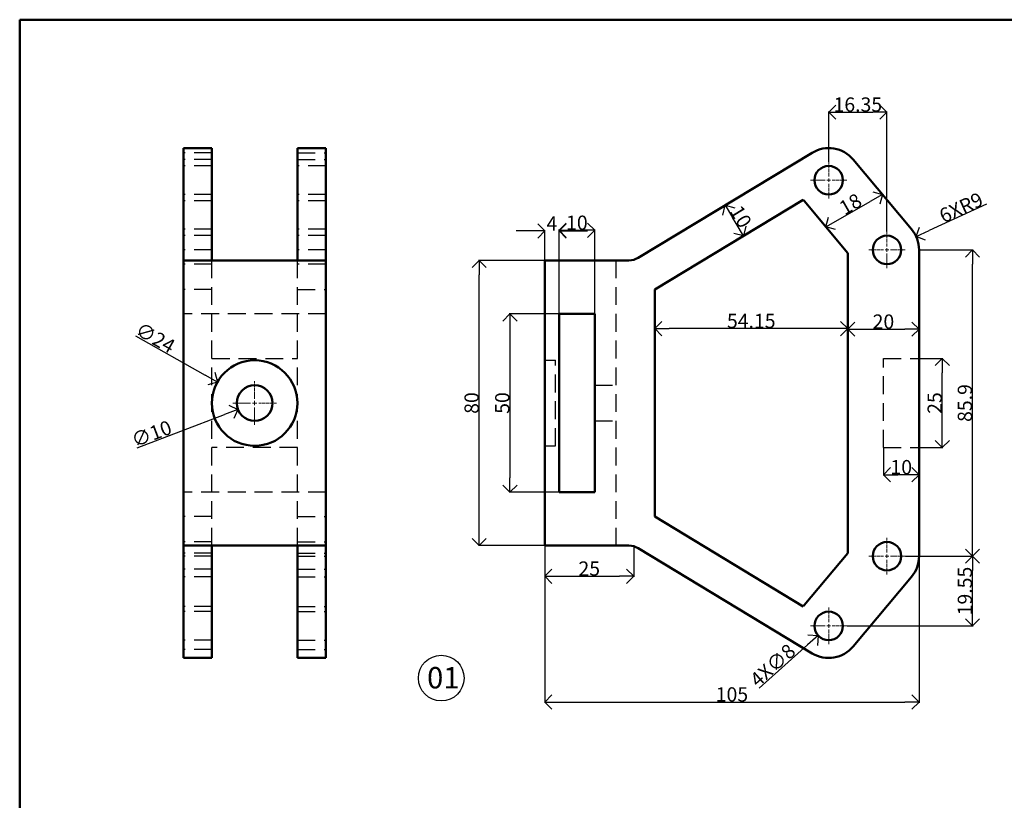
# Model space of a CAD drawing. Units: millimetres. Extents: x 45 to 546, y 51 to 638.
# Tile 3 of 4: x 45 to 322, y 419 to 638. Entities that reach past the tile are written whole.
import ezdxf

# ---------------------------------------------------------------- set-up
doc = ezdxf.new("R2010")
doc.units = ezdxf.units.MM
doc.header["$MEASUREMENT"] = 0
doc.linetypes.add('CENTER2', pattern=[1.125, 0.75, -0.125, 0.125, -0.125])
doc.linetypes.add('HIDDEN', pattern=[0.375, 0.25, -0.125])
for name, color, linetype, lineweight in [('M-CNTR', 1, 'CENTER2', 18), ('M-DIMS', 2, 'Continuous', 25), ('M-HIDN', 8, 'HIDDEN', 25), ('M-OUTL', 7, 'Continuous', 50), ('M-TEXT', 7, 'Continuous', 25), ('M-TTLB', 7, 'Continuous', 50)]:
    doc.layers.add(name, color=color, linetype=linetype, lineweight=lineweight)
doc.styles.get("Standard").update_dxf_attribs({"font": 'arial.ttf'})
doc.dimstyles.get("Standard").update_dxf_attribs({"dimtxt": 4, "dimasz": 4, "dimexe": 0.18, "dimexo": 0.0625, "dimgap": 0.09, "dimtad": 1, "dimdec": 0, "dimzin": 0, "dimdsep": 46, "dimtxsty": 'Standard', "dimblk": 'OPEN90', "dimcen": 0.09, "dimclre": 251, "dimadec": 0, "dimazin": 0, "dimtfac": 1, "dimtdec": 0, "dimtofl": 0, "dimtmove": 0, "dimatfit": 3, "dimfxl": 1, "dimtolj": 1, "dimtzin": 0, "dimarcsym": 0})

# ---------------------------------------------------------------- blocks, each defined once
blk = doc.blocks.new('*U4')
at = {"layer": 'M-CNTR', "color": 0, "transparency": 16777216}
for p, q in [((0, 1.2), (0, 6.12)), ((-6.12, 0), (-1.2, 0)), ((1.2, 0), (6.12, 0)), ((0, -6.12), (0, -1.2))]:
    blk.add_line(p, q, dxfattribs=at)
at = {"layer": 'M-CNTR', "color": 0, "linetype": 'Continuous', "transparency": 16777216}
for p, q in [((-0.6, 0), (0.6, 0)), ((0, -0.6), (0, 0.6))]:
    blk.add_line(p, q, dxfattribs=at)
blk = doc.blocks.new('*U5')
at = {"layer": 'M-CNTR', "color": 0, "transparency": 16777216}
for p, q in [((0, 1), (0, 5.12)), ((-5.12, 0), (-1, 0)), ((1, 0), (5.12, 0)), ((0, -5.12), (0, -1))]:
    blk.add_line(p, q, dxfattribs=at)
at = {"layer": 'M-CNTR', "color": 0, "linetype": 'Continuous', "transparency": 16777216}
for p, q in [((-0.5, 0), (0.5, 0)), ((0, -0.5), (0, 0.5))]:
    blk.add_line(p, q, dxfattribs=at)
blk = doc.blocks.new('*U6')
at = {"layer": 'M-CNTR', "color": 0, "transparency": 16777216}
for p, q in [((0, 1), (0, 5.12)), ((-5.12, 0), (-1, 0)), ((1, 0), (5.12, 0)), ((0, -5.12), (0, -1))]:
    blk.add_line(p, q, dxfattribs=at)
at = {"layer": 'M-CNTR', "color": 0, "linetype": 'Continuous', "transparency": 16777216}
for p, q in [((-0.5, 0), (0.5, 0)), ((0, -0.5), (0, 0.5))]:
    blk.add_line(p, q, dxfattribs=at)
blk = doc.blocks.new('*U7')
at = {"layer": 'M-CNTR', "color": 0, "transparency": 16777216}
for p, q in [((0, 1), (0, 5.12)), ((-5.12, 0), (-1, 0)), ((1, 0), (5.12, 0)), ((0, -5.12), (0, -1))]:
    blk.add_line(p, q, dxfattribs=at)
at = {"layer": 'M-CNTR', "color": 0, "linetype": 'Continuous', "transparency": 16777216}
for p, q in [((-0.5, 0), (0.5, 0)), ((0, -0.5), (0, 0.5))]:
    blk.add_line(p, q, dxfattribs=at)
blk = doc.blocks.new('*U8')
at = {"layer": 'M-CNTR', "color": 0, "transparency": 16777216}
for p, q in [((0, 1), (0, 5.12)), ((-5.12, 0), (-1, 0)), ((1, 0), (5.12, 0)), ((0, -5.12), (0, -1))]:
    blk.add_line(p, q, dxfattribs=at)
at = {"layer": 'M-CNTR', "color": 0, "linetype": 'Continuous', "transparency": 16777216}
for p, q in [((-0.5, 0), (0.5, 0)), ((0, -0.5), (0, 0.5))]:
    blk.add_line(p, q, dxfattribs=at)
blk = doc.blocks.new('_Open90')
at = {"color": 0, "linetype": 'ByBlock', "lineweight": -2}
for p, q in [((0, 0), (-1, 0)), ((-0.5, 0.5), (0, 0)), ((0, 0), (-0.5, -0.5))]:
    blk.add_line(p, q, dxfattribs=at)
blk = doc.blocks.new('*D9')
at = {"layer": 'Defpoints', "color": 0, "transparency": 16777216}
for p in [(100.83, 536.27), (121.73, 524.47)]:
    blk.add_point(p, dxfattribs=at)
at = {"layer": 'M-DIMS', "color": 0, "lineweight": -2, "transparency": 16777216}
for p, q in [((77.85, 549.25), (97.35, 538.24)), ((111.28, 530.28), (111.28, 530.46)), ((111.19, 530.37), (111.37, 530.37))]:
    blk.add_line(p, q, dxfattribs=at)
at = {"layer": 'M-DIMS', "color": 0, "lineweight": -2, "transparency": 16777216, "xscale": 4, "yscale": 4, "zscale": 4, "rotation": 330.5336294164444}
blk.add_blockref('_Open90', (100.83, 536.27), dxfattribs=at)
at = {"layer": 'M-DIMS', "color": 0, "transparency": 16777216, "insert": (83.42, 548.69), "char_height": 4, "attachment_point": 5, "rotation": 330.5336}
blk.add_mtext('\\A1;∅24', dxfattribs=at)
blk = doc.blocks.new('*D10')
at = {"layer": 'Defpoints', "color": 0, "transparency": 16777216}
for p in [(115.95, 532.14), (106.6, 528.59)]:
    blk.add_point(p, dxfattribs=at)
at = {"layer": 'M-DIMS', "color": 0, "lineweight": -2, "transparency": 16777216}
for p, q in [((111.28, 530.28), (111.28, 530.46)), ((111.19, 530.37), (111.37, 530.37)), ((78.35, 517.86), (102.86, 527.17))]:
    blk.add_line(p, q, dxfattribs=at)
at = {"layer": 'M-DIMS', "color": 0, "lineweight": -2, "transparency": 16777216, "xscale": 4, "yscale": 4, "zscale": 4, "rotation": 20.80031859419077}
blk.add_blockref('_Open90', (106.6, 528.59), dxfattribs=at)
at = {"layer": 'M-DIMS', "color": 0, "transparency": 16777216, "insert": (82.34, 521.78), "char_height": 4, "attachment_point": 5, "rotation": 20.8003}
blk.add_mtext('\\A1;∅10', dxfattribs=at)
blk = doc.blocks.new('*D11')
at = {"layer": 'Defpoints', "color": 0, "transparency": 16777216}
for p in [(174.27, 570.38), (192.68, 570.38), (192.68, 490.38)]:
    blk.add_point(p, dxfattribs=at)
at = {"layer": 'M-DIMS', "color": 0, "lineweight": -2, "transparency": 16777216}
for p, q in [((192.61, 570.38), (174.09, 570.38)), ((174.27, 494.38), (174.27, 566.38)), ((192.61, 490.38), (174.09, 490.38))]:
    blk.add_line(p, q, dxfattribs=at)
at = {"layer": 'M-DIMS', "color": 0, "lineweight": -2, "transparency": 16777216, "xscale": 4, "yscale": 4, "zscale": 4}
for p, rotation in [((174.27, 570.38), 90), ((174.27, 490.38), 270)]:
    blk.add_blockref('_Open90', p, dxfattribs=dict(at, rotation=rotation))
at = {"layer": 'M-DIMS', "color": 0, "transparency": 16777216, "insert": (172.14, 530.38), "char_height": 4, "attachment_point": 5, "rotation": 90}
blk.add_mtext('\\A1;80', dxfattribs=at)
blk = doc.blocks.new('*D12')
at = {"layer": 'Defpoints', "color": 0, "transparency": 16777216}
for p in [(196.68, 555.38), (182.88, 505.38), (196.68, 505.38)]:
    blk.add_point(p, dxfattribs=at)
at = {"layer": 'M-DIMS', "color": 0, "lineweight": -2, "transparency": 16777216}
for p, q in [((196.61, 555.38), (182.7, 555.38)), ((182.88, 551.38), (182.88, 509.38)), ((196.61, 505.38), (182.7, 505.38))]:
    blk.add_line(p, q, dxfattribs=at)
at = {"layer": 'M-DIMS', "color": 0, "lineweight": -2, "transparency": 16777216, "xscale": 4, "yscale": 4, "zscale": 4}
for p, rotation in [((182.88, 555.38), 90), ((182.88, 505.38), 270)]:
    blk.add_blockref('_Open90', p, dxfattribs=dict(at, rotation=rotation))
at = {"layer": 'M-DIMS', "color": 0, "transparency": 16777216, "insert": (180.75, 530.38), "char_height": 4, "attachment_point": 5, "rotation": 90}
blk.add_mtext('\\A1;50', dxfattribs=at)
blk = doc.blocks.new('*D13')
at = {"layer": 'Defpoints', "color": 0, "transparency": 16777216}
for p in [(192.68, 578.65), (192.68, 570.38), (196.68, 555.38)]:
    blk.add_point(p, dxfattribs=at)
at = {"layer": 'M-DIMS', "color": 0, "lineweight": -2, "transparency": 16777216}
for p, q in [((188.68, 578.65), (184.68, 578.65)), ((192.68, 570.44), (192.68, 578.83)), ((196.68, 555.44), (196.68, 578.83)), ((200.68, 578.65), (204.68, 578.65))]:
    blk.add_line(p, q, dxfattribs=at)
at = {"layer": 'M-DIMS', "color": 0, "lineweight": -2, "transparency": 16777216, "xscale": 4, "yscale": 4, "zscale": 4}
blk.add_blockref('_Open90', (192.68, 578.65), dxfattribs=at)
at = {"layer": 'M-DIMS', "color": 0, "lineweight": -2, "transparency": 16777216, "xscale": 4, "yscale": 4, "zscale": 4, "rotation": 180}
blk.add_blockref('_Open90', (196.68, 578.65), dxfattribs=at)
at = {"layer": 'M-DIMS', "color": 0, "transparency": 16777216, "insert": (194.68, 580.74), "char_height": 4, "attachment_point": 5}
blk.add_mtext('\\A1;4', dxfattribs=at)
blk = doc.blocks.new('*D14')
at = {"layer": 'Defpoints', "color": 0, "transparency": 16777216}
for p in [(206.68, 578.83), (196.68, 555.38), (206.68, 555.38)]:
    blk.add_point(p, dxfattribs=at)
at = {"layer": 'M-DIMS', "color": 0, "lineweight": -2, "transparency": 16777216}
for p, q in [((196.68, 555.44), (196.68, 579.01)), ((200.68, 578.83), (202.68, 578.83)), ((206.68, 555.44), (206.68, 579.01))]:
    blk.add_line(p, q, dxfattribs=at)
at = {"layer": 'M-DIMS', "color": 0, "lineweight": -2, "transparency": 16777216, "xscale": 4, "yscale": 4, "zscale": 4, "rotation": 180}
blk.add_blockref('_Open90', (196.68, 578.83), dxfattribs=at)
at = {"layer": 'M-DIMS', "color": 0, "lineweight": -2, "transparency": 16777216, "xscale": 4, "yscale": 4, "zscale": 4}
blk.add_blockref('_Open90', (206.68, 578.83), dxfattribs=at)
at = {"layer": 'M-DIMS', "color": 0, "transparency": 16777216, "insert": (201.68, 580.96), "char_height": 4, "attachment_point": 5}
blk.add_mtext('\\A1;10', dxfattribs=at)
blk = doc.blocks.new('*D15')
at = {"layer": 'Defpoints', "color": 0, "transparency": 16777216}
for p in [(288.68, 611.96), (272.33, 598), (288.68, 578.45)]:
    blk.add_point(p, dxfattribs=at)
at = {"layer": 'M-DIMS', "color": 0, "lineweight": -2, "transparency": 16777216}
for p, q in [((272.33, 598.06), (272.33, 612.14)), ((276.33, 611.96), (284.68, 611.96)), ((288.68, 578.51), (288.68, 612.14))]:
    blk.add_line(p, q, dxfattribs=at)
at = {"layer": 'M-DIMS', "color": 0, "lineweight": -2, "transparency": 16777216, "xscale": 4, "yscale": 4, "zscale": 4, "rotation": 180}
blk.add_blockref('_Open90', (272.33, 611.96), dxfattribs=at)
at = {"layer": 'M-DIMS', "color": 0, "lineweight": -2, "transparency": 16777216, "xscale": 4, "yscale": 4, "zscale": 4}
blk.add_blockref('_Open90', (288.68, 611.96), dxfattribs=at)
at = {"layer": 'M-DIMS', "color": 0, "transparency": 16777216, "insert": (280.5, 614.1), "char_height": 4, "attachment_point": 5}
blk.add_mtext('\\A1;16.35', dxfattribs=at)
blk = doc.blocks.new('*D16')
at = {"layer": 'Defpoints', "color": 0, "transparency": 16777216}
for p in [(243.27, 585.84), (241.76, 584.92), (246.93, 576.36)]:
    blk.add_point(p, dxfattribs=at)
at = {"layer": 'M-DIMS', "color": 0, "lineweight": -2, "transparency": 16777216}
for p, q in [((241.81, 584.96), (243.42, 585.93)), ((246.37, 580.7), (245.34, 582.41)), ((246.98, 576.4), (248.6, 577.37))]:
    blk.add_line(p, q, dxfattribs=at)
at = {"layer": 'M-DIMS', "color": 0, "lineweight": -2, "transparency": 16777216, "xscale": 4, "yscale": 4, "zscale": 4}
for p, rotation in [((243.27, 585.84), 121.1367457519999), ((248.44, 577.28), 301.136745752)]:
    blk.add_blockref('_Open90', p, dxfattribs=dict(at, rotation=rotation))
at = {"layer": 'M-DIMS', "color": 0, "transparency": 16777216, "insert": (247.68, 582.66), "char_height": 4, "attachment_point": 5, "rotation": 301.1367}
blk.add_mtext('\\A1;10', dxfattribs=at)
blk = doc.blocks.new('*D17')
at = {"layer": 'Defpoints', "color": 0, "transparency": 16777216}
for p in [(287.4, 588.88), (287.4, 588.88), (271.55, 579.78)]:
    blk.add_point(p, dxfattribs=at)
at = {"layer": 'M-DIMS', "color": 0, "lineweight": -2, "transparency": 16777216}
for p, q in [((287.44, 588.82), (287.49, 588.72)), ((275.02, 581.77), (283.94, 586.88)), ((271.58, 579.72), (271.64, 579.62))]:
    blk.add_line(p, q, dxfattribs=at)
at = {"layer": 'M-DIMS', "color": 0, "lineweight": -2, "transparency": 16777216, "xscale": 4, "yscale": 4, "zscale": 4}
for p, rotation in [((287.4, 588.88), 29.84897271971798), ((271.55, 579.78), 209.848972719718)]:
    blk.add_blockref('_Open90', p, dxfattribs=dict(at, rotation=rotation))
at = {"layer": 'M-DIMS', "color": 0, "transparency": 16777216, "insert": (278.42, 586.18), "char_height": 4, "attachment_point": 5, "rotation": 29.849}
blk.add_mtext('\\A1;18', dxfattribs=at)
blk = doc.blocks.new('*D18')
at = {"layer": 'Defpoints', "color": 0, "transparency": 16777216}
for p in [(192.68, 490.38), (217.62, 490.19), (217.62, 481.81)]:
    blk.add_point(p, dxfattribs=at)
at = {"layer": 'M-DIMS', "color": 0, "lineweight": -2, "transparency": 16777216}
for p, q in [((192.68, 490.31), (192.68, 481.63)), ((217.62, 490.13), (217.62, 481.63)), ((196.68, 481.81), (213.62, 481.81))]:
    blk.add_line(p, q, dxfattribs=at)
at = {"layer": 'M-DIMS', "color": 0, "lineweight": -2, "transparency": 16777216, "xscale": 4, "yscale": 4, "zscale": 4, "rotation": 180}
blk.add_blockref('_Open90', (192.68, 481.81), dxfattribs=at)
at = {"layer": 'M-DIMS', "color": 0, "lineweight": -2, "transparency": 16777216, "xscale": 4, "yscale": 4, "zscale": 4}
blk.add_blockref('_Open90', (217.62, 481.81), dxfattribs=at)
at = {"layer": 'M-DIMS', "color": 0, "transparency": 16777216, "insert": (205.15, 483.95), "char_height": 4, "attachment_point": 5}
blk.add_mtext('\\A1;25', dxfattribs=at)
blk = doc.blocks.new('*D19')
at = {"layer": 'Defpoints', "color": 0, "transparency": 16777216}
for p in [(192.68, 490.38), (297.68, 487.43), (297.68, 446.52)]:
    blk.add_point(p, dxfattribs=at)
at = {"layer": 'M-DIMS', "color": 0, "lineweight": -2, "transparency": 16777216}
for p, q in [((192.68, 490.31), (192.68, 446.34)), ((297.68, 487.36), (297.68, 446.34)), ((196.68, 446.52), (293.68, 446.52))]:
    blk.add_line(p, q, dxfattribs=at)
at = {"layer": 'M-DIMS', "color": 0, "lineweight": -2, "transparency": 16777216, "xscale": 4, "yscale": 4, "zscale": 4, "rotation": 180}
blk.add_blockref('_Open90', (192.68, 446.52), dxfattribs=at)
at = {"layer": 'M-DIMS', "color": 0, "lineweight": -2, "transparency": 16777216, "xscale": 4, "yscale": 4, "zscale": 4}
blk.add_blockref('_Open90', (297.68, 446.52), dxfattribs=at)
at = {"layer": 'M-DIMS', "color": 0, "transparency": 16777216, "insert": (245.18, 448.65), "char_height": 4, "attachment_point": 5}
blk.add_mtext('\\A1;105', dxfattribs=at)
blk = doc.blocks.new('*D20')
at = {"layer": 'Defpoints', "color": 0, "transparency": 16777216}
for p in [(293.8, 487.43), (312.66, 487.43), (277.45, 467.88)]:
    blk.add_point(p, dxfattribs=at)
at = {"layer": 'M-DIMS', "color": 0, "lineweight": -2, "transparency": 16777216}
for p, q in [((293.86, 487.43), (312.84, 487.43)), ((312.66, 471.88), (312.66, 483.43)), ((277.51, 467.88), (312.84, 467.88))]:
    blk.add_line(p, q, dxfattribs=at)
at = {"layer": 'M-DIMS', "color": 0, "lineweight": -2, "transparency": 16777216, "xscale": 4, "yscale": 4, "zscale": 4}
for p, rotation in [((312.66, 487.43), 90), ((312.66, 467.88), 270)]:
    blk.add_blockref('_Open90', p, dxfattribs=dict(at, rotation=rotation))
at = {"layer": 'M-DIMS', "color": 0, "transparency": 16777216, "insert": (310.53, 477.65), "char_height": 4, "attachment_point": 5, "rotation": 90}
blk.add_mtext('\\A1;19.55', dxfattribs=at)
blk = doc.blocks.new('*D21')
at = {"layer": 'Defpoints', "color": 0, "transparency": 16777216}
for p in [(297.68, 573.33), (312.66, 573.33), (297.68, 487.43)]:
    blk.add_point(p, dxfattribs=at)
at = {"layer": 'M-DIMS', "color": 0, "lineweight": -2, "transparency": 16777216}
for p, q in [((297.74, 573.33), (312.84, 573.33)), ((312.66, 491.43), (312.66, 569.33)), ((297.74, 487.43), (312.84, 487.43))]:
    blk.add_line(p, q, dxfattribs=at)
at = {"layer": 'M-DIMS', "color": 0, "lineweight": -2, "transparency": 16777216, "xscale": 4, "yscale": 4, "zscale": 4}
for p, rotation in [((312.66, 573.33), 90), ((312.66, 487.43), 270)]:
    blk.add_blockref('_Open90', p, dxfattribs=dict(at, rotation=rotation))
at = {"layer": 'M-DIMS', "color": 0, "transparency": 16777216, "insert": (310.53, 530.38), "char_height": 4, "attachment_point": 5, "rotation": 90}
blk.add_mtext('\\A1;85.9', dxfattribs=at)
blk = doc.blocks.new('*D22')
at = {"layer": 'Defpoints', "color": 0, "transparency": 16777216}
for p in [(297.68, 542.88), (304.19, 542.88), (297.68, 517.88)]:
    blk.add_point(p, dxfattribs=at)
at = {"layer": 'M-DIMS', "color": 0, "lineweight": -2, "transparency": 16777216}
for p, q in [((297.74, 542.88), (304.37, 542.88)), ((304.19, 521.88), (304.19, 538.88)), ((297.74, 517.88), (304.37, 517.88))]:
    blk.add_line(p, q, dxfattribs=at)
at = {"layer": 'M-DIMS', "color": 0, "lineweight": -2, "transparency": 16777216, "xscale": 4, "yscale": 4, "zscale": 4}
for p, rotation in [((304.19, 542.88), 90), ((304.19, 517.88), 270)]:
    blk.add_blockref('_Open90', p, dxfattribs=dict(at, rotation=rotation))
at = {"layer": 'M-DIMS', "color": 0, "transparency": 16777216, "insert": (302.06, 530.38), "char_height": 4, "attachment_point": 5, "rotation": 90}
blk.add_mtext('\\A1;25', dxfattribs=at)
blk = doc.blocks.new('*D23')
at = {"layer": 'Defpoints', "color": 0, "transparency": 16777216}
for p in [(287.68, 517.88), (297.68, 517.88), (287.68, 510.27)]:
    blk.add_point(p, dxfattribs=at)
at = {"layer": 'M-DIMS', "color": 0, "lineweight": -2, "transparency": 16777216}
for p, q in [((287.68, 517.81), (287.68, 510.09)), ((297.68, 517.81), (297.68, 510.09)), ((293.68, 510.27), (291.68, 510.27))]:
    blk.add_line(p, q, dxfattribs=at)
at = {"layer": 'M-DIMS', "color": 0, "lineweight": -2, "transparency": 16777216, "xscale": 4, "yscale": 4, "zscale": 4, "rotation": 180}
blk.add_blockref('_Open90', (287.68, 510.27), dxfattribs=at)
at = {"layer": 'M-DIMS', "color": 0, "lineweight": -2, "transparency": 16777216, "xscale": 4, "yscale": 4, "zscale": 4}
blk.add_blockref('_Open90', (297.68, 510.27), dxfattribs=at)
at = {"layer": 'M-DIMS', "color": 0, "transparency": 16777216, "insert": (292.68, 512.4), "char_height": 4, "attachment_point": 5}
blk.add_mtext('\\A1;10', dxfattribs=at)
blk = doc.blocks.new('*D24')
at = {"layer": 'Defpoints', "color": 0, "transparency": 16777216}
for p in [(277.68, 551.09), (297.68, 551.09), (297.68, 551.09)]:
    blk.add_point(p, dxfattribs=at)
at = {"layer": 'M-DIMS', "color": 0, "lineweight": -2, "transparency": 16777216}
for p, q in [((277.68, 551.15), (277.68, 551.27)), ((281.68, 551.09), (293.68, 551.09)), ((297.68, 551.15), (297.68, 551.27))]:
    blk.add_line(p, q, dxfattribs=at)
at = {"layer": 'M-DIMS', "color": 0, "lineweight": -2, "transparency": 16777216, "xscale": 4, "yscale": 4, "zscale": 4, "rotation": 180}
blk.add_blockref('_Open90', (277.68, 551.09), dxfattribs=at)
at = {"layer": 'M-DIMS', "color": 0, "lineweight": -2, "transparency": 16777216, "xscale": 4, "yscale": 4, "zscale": 4}
blk.add_blockref('_Open90', (297.68, 551.09), dxfattribs=at)
at = {"layer": 'M-DIMS', "color": 0, "transparency": 16777216, "insert": (287.68, 553.22), "char_height": 4, "attachment_point": 5}
blk.add_mtext('\\A1;20', dxfattribs=at)
blk = doc.blocks.new('*D25')
at = {"layer": 'Defpoints', "color": 0, "transparency": 16777216}
for p in [(223.53, 551.27), (223.53, 551.27), (277.68, 551.27)]:
    blk.add_point(p, dxfattribs=at)
at = {"layer": 'M-DIMS', "color": 0, "lineweight": -2, "transparency": 16777216}
for p, q in [((223.53, 551.33), (223.53, 551.45)), ((273.68, 551.27), (227.53, 551.27)), ((277.68, 551.33), (277.68, 551.45))]:
    blk.add_line(p, q, dxfattribs=at)
at = {"layer": 'M-DIMS', "color": 0, "lineweight": -2, "transparency": 16777216, "xscale": 4, "yscale": 4, "zscale": 4, "rotation": 180}
blk.add_blockref('_Open90', (223.53, 551.27), dxfattribs=at)
at = {"layer": 'M-DIMS', "color": 0, "lineweight": -2, "transparency": 16777216, "xscale": 4, "yscale": 4, "zscale": 4}
blk.add_blockref('_Open90', (277.68, 551.27), dxfattribs=at)
at = {"layer": 'M-DIMS', "color": 0, "transparency": 16777216, "insert": (250.6, 553.4), "char_height": 4, "attachment_point": 5}
blk.add_mtext('\\A1;54.15', dxfattribs=at)
blk = doc.blocks.new('*D26')
at = {"layer": 'Defpoints', "color": 0, "transparency": 16777216}
for p in [(296.86, 577.08), (288.68, 573.33)]:
    blk.add_point(p, dxfattribs=at)
at = {"layer": 'M-DIMS', "color": 0, "lineweight": -2, "transparency": 16777216}
for p, q in [((316.58, 586.12), (300.49, 578.74)), ((288.59, 573.33), (288.77, 573.33)), ((288.68, 573.24), (288.68, 573.42))]:
    blk.add_line(p, q, dxfattribs=at)
at = {"layer": 'M-DIMS', "color": 0, "lineweight": -2, "transparency": 16777216, "xscale": 4, "yscale": 4, "zscale": 4, "rotation": 204.6310426737453}
blk.add_blockref('_Open90', (296.86, 577.08), dxfattribs=at)
at = {"layer": 'M-DIMS', "color": 0, "transparency": 16777216, "insert": (309.47, 585.21), "char_height": 4, "attachment_point": 5, "rotation": 24.631}
blk.add_mtext('\\A1;6XR9', dxfattribs=at)
blk = doc.blocks.new('*D27')
at = {"layer": 'Defpoints', "color": 0, "transparency": 16777216}
for p in [(275.31, 470.54), (269.34, 465.21)]:
    blk.add_point(p, dxfattribs=at)
at = {"layer": 'M-DIMS', "color": 0, "lineweight": -2, "transparency": 16777216}
for p, q in [((272.24, 467.88), (272.42, 467.88)), ((272.33, 467.79), (272.33, 467.97)), ((252.83, 450.44), (266.36, 462.54))]:
    blk.add_line(p, q, dxfattribs=at)
at = {"layer": 'M-DIMS', "color": 0, "lineweight": -2, "transparency": 16777216, "xscale": 4, "yscale": 4, "zscale": 4, "rotation": 41.80963978191437}
blk.add_blockref('_Open90', (269.34, 465.21), dxfattribs=at)
at = {"layer": 'M-DIMS', "color": 0, "transparency": 16777216, "insert": (256.61, 456.83), "char_height": 4, "attachment_point": 5, "rotation": 41.8096}
blk.add_mtext('\\A1;4X∅8', dxfattribs=at)

msp = doc.modelspace()

# ---------------------------------------------------------------- linework, layer by layer
at = {"layer": 'M-HIDN', "ltscale": 20}
for p, q in [((99.277, 600.58), (91.277, 600.58)), ((123.277, 600.58), (131.277, 600.58)), ((99.277, 598.65), (91.277, 598.65)), ((99.277, 596.876), (91.277, 596.876)), ((123.277, 598.65), (131.277, 598.65)), ((131.277, 596.876), (123.277, 596.876)), ((99.277, 588.876), (91.277, 588.876)), ((131.277, 588.876), (123.277, 588.876)), ((99.277, 587.102), (91.277, 587.102)), ((131.277, 587.102), (123.277, 587.102)), ((99.277, 579.1), (91.277, 579.1)), ((131.277, 579.1), (123.277, 579.1)), ((99.277, 577.326), (91.277, 577.326)), ((131.277, 577.326), (123.277, 577.326)), ((99.277, 573.326), (91.277, 573.326)), ((131.277, 573.326), (123.277, 573.326)), ((99.277, 569.326), (91.277, 569.326)), ((99.277, 490.376), (99.277, 570.376)), ((123.277, 490.376), (123.277, 570.376)), ((131.277, 569.326), (123.277, 569.326)), ((212.676, 490.376), (212.676, 570.376)), ((99.277, 562.227), (91.277, 562.227)), ((123.277, 562.227), (131.277, 562.227)), ((131.277, 555.376), (91.277, 555.376)), ((99.277, 542.876), (123.277, 542.876)), ((192.676, 542.376), (195.676, 542.376)), ((195.676, 518.376), (195.676, 542.376)), ((287.676, 542.876), (297.676, 542.876)), ((287.676, 517.876), (287.676, 542.876)), ((206.676, 535.376), (212.676, 535.376)), ((206.676, 525.376), (212.676, 525.376)), ((123.277, 517.876), (99.277, 517.876)), ((192.676, 518.376), (195.676, 518.376)), ((287.676, 517.876), (297.676, 517.876)), ((131.277, 505.376), (91.277, 505.376)), ((99.277, 498.525), (91.277, 498.525)), ((123.277, 498.525), (131.277, 498.525)), ((99.277, 491.426), (91.277, 491.426)), ((123.277, 491.426), (131.277, 491.426)), ((99.277, 488.302), (91.277, 488.302)), ((99.277, 487.426), (91.277, 487.426)), ((123.277, 488.302), (131.277, 488.302)), ((123.277, 487.426), (131.277, 487.426)), ((99.277, 483.825), (91.277, 483.825)), ((123.277, 483.825), (131.277, 483.825)), ((99.277, 481.652), (91.277, 481.652)), ((123.277, 481.652), (131.277, 481.652)), ((99.277, 473.357), (91.277, 473.357)), ((123.277, 473.357), (131.277, 473.357)), ((99.277, 471.876), (91.277, 471.876)), ((123.277, 471.876), (131.277, 471.876)), ((99.277, 463.876), (91.277, 463.876)), ((123.277, 463.876), (131.277, 463.876)), ((99.277, 461.242), (91.277, 461.242)), ((123.277, 461.242), (131.277, 461.242))]:
    msp.add_line(p, q, dxfattribs=at)
at = {"layer": 'M-OUTL'}
for p, q in [((91.277, 601.862), (99.277, 601.862)), ((91.277, 458.876), (91.277, 601.862)), ((99.277, 570.376), (99.277, 601.862)), ((123.277, 601.862), (131.277, 601.862)), ((123.277, 570.376), (123.277, 601.862)), ((131.277, 458.876), (131.277, 601.862)), ((218.868, 571.097), (267.672, 600.58)), ((295.58, 579.1), (279.23, 598.65)), ((223.526, 562.227), (265.187, 587.395)), ((277.676, 572.45), (265.422, 587.102)), ((277.676, 488.302), (277.676, 572.45)), ((297.676, 487.426), (297.676, 573.326)), ((131.277, 570.376), (91.277, 570.376)), ((192.676, 490.376), (192.676, 570.376)), ((192.676, 570.376), (216.283, 570.376)), ((223.526, 498.525), (223.526, 562.227)), ((196.676, 505.376), (196.676, 555.376)), ((196.676, 555.376), (206.676, 555.376)), ((206.676, 505.376), (206.676, 555.376)), ((196.676, 505.376), (206.676, 505.376)), ((223.526, 498.525), (265.187, 473.357)), ((131.277, 490.376), (91.277, 490.376)), ((99.277, 458.876), (99.277, 490.376)), ((123.277, 458.876), (123.277, 490.376)), ((192.676, 490.376), (216.283, 490.376)), ((218.868, 489.656), (267.672, 460.173)), ((265.422, 473.65), (277.676, 488.302)), ((279.23, 462.102), (295.58, 481.652)), ((99.277, 458.876), (91.277, 458.876)), ((123.277, 458.876), (131.277, 458.876))]:
    msp.add_line(p, q, dxfattribs=at)
for centre, radius in [((272.326, 592.876), 4), ((288.676, 573.326), 4), ((111.277, 530.369), 12), ((111.277, 530.369), 5), ((288.676, 487.426), 4), ((272.326, 467.876), 4)]:
    msp.add_circle(centre, radius, dxfattribs=at)
for centre, radius, start, end in [((272.326, 592.876), 9, 39.90632, 121.13675), ((272.326, 592.876), 9, 217.51612, 219.90632), ((288.676, 573.326), 9, 0, 39.90632), ((216.283, 575.376), 5, 270, 301.13675), ((216.283, 485.376), 5, 58.86325, 90), ((288.676, 487.426), 9, 320.09368, 0), ((272.326, 467.876), 9, 140.09368, 142.48388), ((272.326, 467.876), 9, 238.86325, 320.09368)]:
    msp.add_arc(centre, radius, start, end, dxfattribs=at)
at = {"layer": 'M-TEXT'}
msp.add_circle((163.631, 453.239), 6.408, dxfattribs=at)
at = {"layer": 'M-TTLB'}
msp.add_lwpolyline([(45.357, 637.893), (546.237, 637.893), (546.237, 51.054), (45.357, 51.054)], close=True, dxfattribs=at)

# ---------------------------------------------------------------- block references
at = {"layer": 'M-CNTR'}
for name, p in [('*U8', (272.326, 592.876)), ('*U7', (288.676, 573.326)), ('*U4', (111.277, 530.369)), ('*U6', (288.676, 487.426)), ('*U5', (272.326, 467.876))]:
    msp.add_blockref(name, p, dxfattribs=at)

# ---------------------------------------------------------------- texts
at = {"layer": 'M-TEXT', "insert": (159.652, 456.335), "char_height": 6, "attachment_point": 1}
msp.add_mtext_dynamic_manual_height_columns('01', width=105.49417, gutter_width=1, heights=[0], dxfattribs=at)

# ---------------------------------------------------------------- dimensions: what is measured, and where the dimension line sits
at = {"layer": 'M-DIMS'}
for base, p1, p2, override, picture, middle in [((288.676, 611.962), (272.326, 597.996), (288.676, 578.446), {"dimdec": 2, "dimclrd": 0, "dimclre": 0, "dimclrt": 0}, '*D15', (280.501, 614.095)), ((192.676, 578.653), (196.676, 555.376), (192.676, 570.376), {"dimclrd": 0, "dimclre": 0, "dimclrt": 0}, '*D13', (194.676, 580.743)), ((206.676, 578.833), (196.676, 555.376), (206.676, 555.376), {"dimclrd": 0, "dimclre": 0, "dimclrt": 0}, '*D14', (201.676, 580.965)), ((223.526, 551.269), (277.676, 551.269), (223.526, 551.269), {"dimdec": 2, "dimclrd": 0, "dimclre": 0, "dimclrt": 0}, '*D25', (250.601, 553.402)), ((297.676, 551.089), (277.676, 551.089), (297.676, 551.089), {"dimclrd": 0, "dimclre": 0, "dimclrt": 0}, '*D24', (287.676, 553.222)), ((287.676, 510.267), (297.676, 517.876), (287.676, 517.876), {"dimclrd": 0, "dimclre": 0, "dimclrt": 0}, '*D23', (292.676, 512.4)), ((217.625, 481.814), (192.676, 490.376), (217.625, 490.193), {"dimclrd": 0, "dimclre": 0, "dimclrt": 0}, '*D18', (205.151, 483.946)), ((297.676, 446.521), (192.676, 490.376), (297.676, 487.426), {"dimclrd": 0, "dimclre": 0, "dimclrt": 0}, '*D19', (245.176, 448.654))]:
    dim = msp.add_linear_dim(base=base, p1=p1, p2=p2, dimstyle='Standard', override=override, dxfattribs=at)
    dim.commit()
    dim.dimension.update_dxf_attribs({"geometry": picture, "text_midpoint": middle})
for p1, p2, distance, picture, middle in [((271.549, 579.776), (287.405, 588.875), 0, '*D17', (278.416, 586.175)), ((246.927, 576.364), (241.756, 584.923), -1.77, '*D16', (247.681, 582.661))]:
    dim = msp.add_aligned_dim(p1=p1, p2=p2, distance=distance, dimstyle='Standard', override={"dimclrd": 0, "dimclre": 0, "dimclrt": 0}, dxfattribs=at)
    dim.commit()
    dim.dimension.update_dxf_attribs({"geometry": picture, "text_midpoint": middle})
dim = msp.add_radius_dim(center=(288.676, 573.326), mpoint=(296.857, 577.077), text='6X<>', dimstyle='Standard', override={"dimclrd": 0, "dimclre": 0, "dimclrt": 0}, dxfattribs=at)
dim.commit()
dim.dimension.update_dxf_attribs({"geometry": '*D26', "text_midpoint": (309.468, 585.205)})
for base, p1, p2, override, picture, middle in [((312.658, 573.326), (297.676, 487.426), (297.676, 573.326), {"dimdec": 1, "dimclrd": 0, "dimclre": 0, "dimclrt": 0}, '*D21', (310.526, 530.376)), ((174.273, 570.376), (192.676, 490.376), (192.676, 570.376), {"dimclrd": 0, "dimclre": 0, "dimclrt": 0}, '*D11', (172.14, 530.376)), ((182.878, 505.376), (196.676, 555.376), (196.676, 505.376), {"dimclrd": 0, "dimclre": 0, "dimclrt": 0}, '*D12', (180.745, 530.376)), ((304.193, 542.876), (297.676, 517.876), (297.676, 542.876), {"dimclrd": 0, "dimclre": 0, "dimclrt": 0}, '*D22', (302.06, 530.376)), ((312.658, 487.426), (277.446, 467.876), (293.796, 487.426), {"dimdec": 2, "dimclrd": 0, "dimclre": 0, "dimclrt": 0}, '*D20', (310.526, 477.651))]:
    dim = msp.add_linear_dim(base=base, p1=p1, p2=p2, angle=90, dimstyle='Standard', override=override, dxfattribs=at)
    dim.commit()
    dim.dimension.update_dxf_attribs({"geometry": picture, "text_midpoint": middle})
for p1, p2, picture, middle in [((121.725, 524.466), (100.83, 536.272), '*D9', (82.312, 546.734)), ((115.952, 532.145), (106.603, 528.593), '*D10', (83.136, 519.679))]:
    dim = msp.add_diameter_dim_2p(p1=p1, p2=p2, dimstyle='Standard', override={"dimclrd": 0, "dimclre": 0, "dimclrt": 0}, dxfattribs=at)
    dim.commit()
    dim.dimension.update_dxf_attribs({"geometry": picture, "text_midpoint": middle, "dimtype": 163})
dim = msp.add_diameter_dim_2p(p1=(275.308, 470.543), p2=(269.345, 465.21), text='4X<>', dimstyle='Standard', override={"dimclrd": 0, "dimclre": 0, "dimclrt": 0}, dxfattribs=at)
dim.commit()
dim.dimension.update_dxf_attribs({"geometry": '*D27', "text_midpoint": (256.611, 456.832)})

doc.saveas('drawing.dxf')
